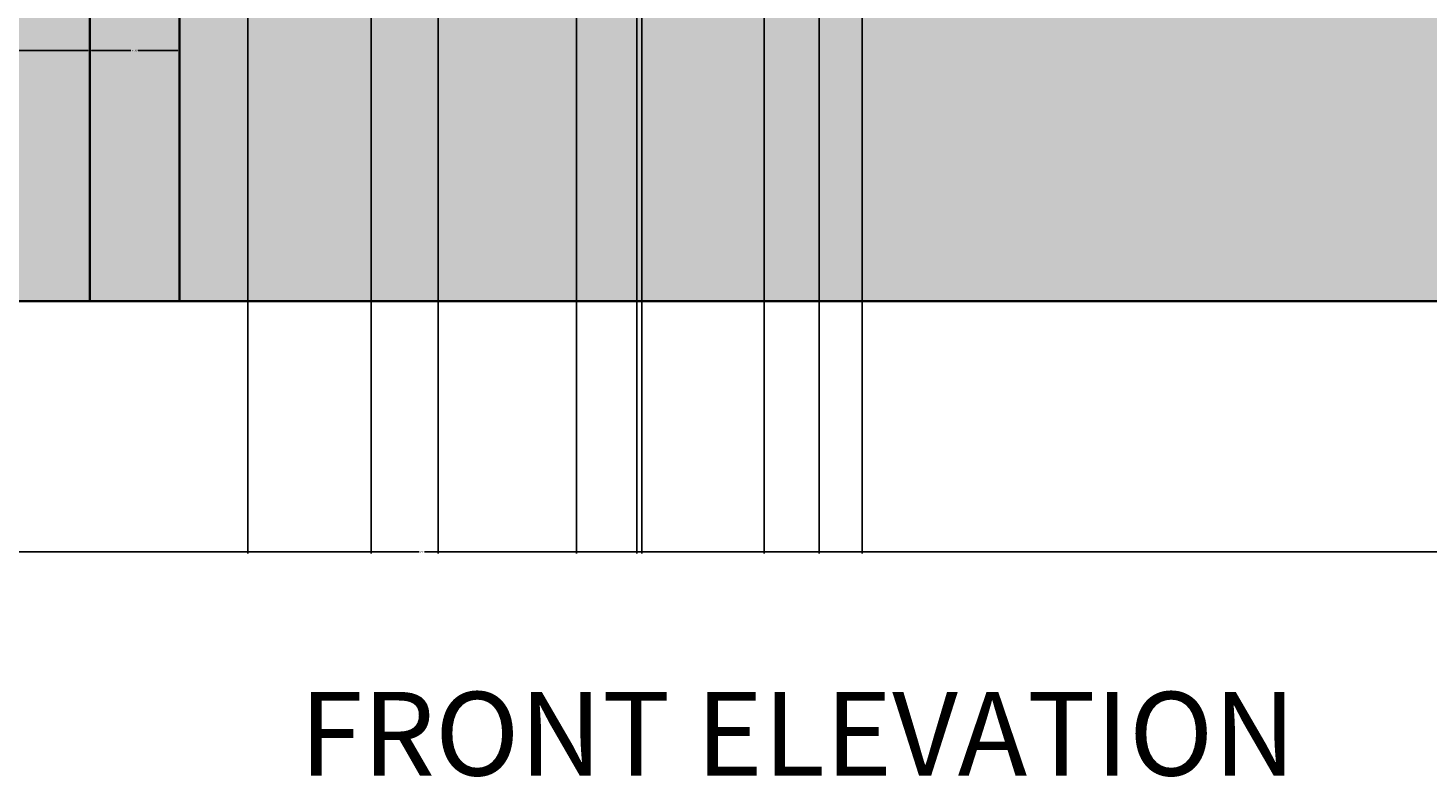
# Model space of a CAD drawing. Units: inches. Extents: x 73 to 607, y 92 to 651.
# Tile 2 of 18: x 298 to 448, y 92 to 173. Entities that reach past the tile are written whole.
import ezdxf

# ---------------------------------------------------------------- set-up
doc = ezdxf.new("R2010")
doc.units = ezdxf.units.IN
doc.header["$MEASUREMENT"] = 0
for name, color, linetype, lineweight in [('A-ANNO-DIMS', 2, 'Continuous', 18), ('A-ANNO-TEXT', 7, 'Continuous', 25), ('A-ELEV', 7, 'Continuous', 35), ('A-ELEV-PATT-WALL', 254, 'Continuous', 13), ('A-ELEV-PATT-WOOD', 32, 'Continuous', 13)]:
    doc.layers.add(name, color=color, linetype=linetype, lineweight=lineweight)
doc.styles.get("Standard").update_dxf_attribs({"font": 'arial.ttf'})
doc.dimstyles.get("Standard").update_dxf_attribs({"dimtxt": 0.18, "dimasz": 0.18, "dimexe": 0.18, "dimexo": 0.0625, "dimgap": 0.09, "dimtad": 0, "dimtih": 1, "dimtoh": 1, "dimdec": 4, "dimzin": 0, "dimdsep": 46, "dimtxsty": 'Standard', "dimcen": 0.09, "dimadec": 0, "dimazin": 0, "dimtfac": 1, "dimtdec": 4, "dimtofl": 0, "dimtmove": 0, "dimatfit": 3, "dimfxl": 1, "dimtolj": 1, "dimtzin": 0, "dimarcsym": 0})

# ---------------------------------------------------------------- blocks, each defined once
blk = doc.blocks.new('*D4')
at = {"layer": 'A-ANNO-DIMS', "color": 0, "lineweight": -2, "transparency": 16777216}
for p, q in [((100.1, 143.14), (100.1, 116.02)), ((580.1, 143.14), (580.1, 116.02)), ((100.28, 116.2), (339.81, 116.2)), ((579.92, 116.2), (340.39, 116.2))]:
    blk.add_line(p, q, dxfattribs=at)
at = {"layer": 'A-ANNO-DIMS', "color": 0, "transparency": 16777216}
for points in [[(100.28, 116.23), (100.28, 116.17), (100.1, 116.2)], [(579.92, 116.23), (579.92, 116.17), (580.1, 116.2)]]:
    blk.add_solid(points, dxfattribs=at)
at = {"layer": 'Defpoints', "color": 0, "transparency": 16777216}
for p in [(100.1, 143.2), (580.1, 143.2), (580.1, 116.2)]:
    blk.add_point(p, dxfattribs=at)
at = {"layer": 'A-ANNO-DIMS', "color": 0, "transparency": 16777216, "insert": (340.1, 116.2), "char_height": 0.18, "attachment_point": 5}
blk.add_mtext('\\A1;480', dxfattribs=at)
blk = doc.blocks.new('*D31')
at = {"layer": 'A-ANNO-DIMS', "color": 0, "lineweight": -2, "transparency": 16777216}
for p, q in [((256.47, 143.27), (256.47, 170.38)), ((304.36, 143.27), (304.36, 170.38)), ((256.65, 170.2), (280.02, 170.2)), ((304.18, 170.2), (280.81, 170.2))]:
    blk.add_line(p, q, dxfattribs=at)
at = {"layer": 'A-ANNO-DIMS', "color": 0, "transparency": 16777216}
for points in [[(256.65, 170.23), (256.65, 170.17), (256.47, 170.2)], [(304.18, 170.23), (304.18, 170.17), (304.36, 170.2)]]:
    blk.add_solid(points, dxfattribs=at)
at = {"layer": 'Defpoints', "color": 0, "transparency": 16777216}
for p in [(304.36, 170.2), (256.47, 143.2), (304.36, 143.2)]:
    blk.add_point(p, dxfattribs=at)
at = {"layer": 'A-ANNO-DIMS', "color": 0, "transparency": 16777216, "insert": (280.41, 170.2), "char_height": 0.18, "attachment_point": 5}
blk.add_mtext('\\A1;47.88', dxfattribs=at)
blk = doc.blocks.new('*D32')
at = {"layer": 'A-ANNO-DIMS', "color": 0, "lineweight": -2, "transparency": 16777216}
for p, q in [((304.36, 143.27), (304.36, 170.38)), ((314.01, 143.27), (314.01, 170.38)), ((304.54, 170.2), (308.79, 170.2)), ((313.83, 170.2), (309.58, 170.2))]:
    blk.add_line(p, q, dxfattribs=at)
at = {"layer": 'A-ANNO-DIMS', "color": 0, "transparency": 16777216}
for points in [[(304.54, 170.23), (304.54, 170.17), (304.36, 170.2)], [(313.83, 170.23), (313.83, 170.17), (314.01, 170.2)]]:
    blk.add_solid(points, dxfattribs=at)
at = {"layer": 'Defpoints', "color": 0, "transparency": 16777216}
for p in [(314.01, 170.2), (304.36, 143.2), (314.01, 143.2)]:
    blk.add_point(p, dxfattribs=at)
at = {"layer": 'A-ANNO-DIMS', "color": 0, "transparency": 16777216, "insert": (309.19, 170.2), "char_height": 0.18, "attachment_point": 5}
blk.add_mtext('\\A1;9.659', dxfattribs=at)
blk = doc.blocks.new('*D77')
at = {"layer": 'A-ANNO-DIMS', "color": 0, "lineweight": -2, "transparency": 16777216}
for p, q in [((321.37, 356.99), (321.37, 116.02)), ((334.67, 320.14), (334.67, 116.02)), ((321.55, 116.2), (327.63, 116.2)), ((334.49, 116.2), (328.4, 116.2))]:
    blk.add_line(p, q, dxfattribs=at)
at = {"layer": 'A-ANNO-DIMS', "color": 0, "transparency": 16777216}
for points in [[(321.55, 116.23), (321.55, 116.17), (321.37, 116.2)], [(334.49, 116.23), (334.49, 116.17), (334.67, 116.2)]]:
    blk.add_solid(points, dxfattribs=at)
at = {"layer": 'Defpoints', "color": 0, "transparency": 16777216}
for p in [(321.37, 357.06), (334.67, 320.2), (321.37, 116.2)]:
    blk.add_point(p, dxfattribs=at)
at = {"layer": 'A-ANNO-DIMS', "color": 0, "transparency": 16777216, "insert": (328.02, 116.2), "char_height": 0.18, "attachment_point": 5}
blk.add_mtext('\\A1;13.30', dxfattribs=at)
blk = doc.blocks.new('*D86')
at = {"layer": 'A-ANNO-DIMS', "color": 0, "lineweight": -2, "transparency": 16777216}
for p, q in [((356.77, 212.97), (356.77, 116.02)), ((341.87, 194.47), (341.87, 116.02)), ((342.05, 116.2), (348.87, 116.2)), ((356.59, 116.2), (349.78, 116.2))]:
    blk.add_line(p, q, dxfattribs=at)
at = {"layer": 'A-ANNO-DIMS', "color": 0, "transparency": 16777216}
for points in [[(342.05, 116.23), (342.05, 116.17), (341.87, 116.2)], [(356.59, 116.23), (356.59, 116.17), (356.77, 116.2)]]:
    blk.add_solid(points, dxfattribs=at)
at = {"layer": 'Defpoints', "color": 0, "transparency": 16777216}
for p in [(356.77, 213.03), (341.87, 194.54), (356.77, 116.2)]:
    blk.add_point(p, dxfattribs=at)
at = {"layer": 'A-ANNO-DIMS', "color": 0, "transparency": 16777216, "insert": (349.32, 116.2), "char_height": 0.18, "attachment_point": 5}
blk.add_mtext('\\A1;14.906', dxfattribs=at)
blk = doc.blocks.new('*D87')
at = {"layer": 'A-ANNO-DIMS', "color": 0, "lineweight": -2, "transparency": 16777216}
for p, q in [((356.77, 212.97), (356.77, 116.02)), ((363.26, 199.09), (363.26, 116.02)), ((356.95, 116.2), (359.62, 116.2)), ((363.08, 116.2), (360.41, 116.2))]:
    blk.add_line(p, q, dxfattribs=at)
at = {"layer": 'A-ANNO-DIMS', "color": 0, "transparency": 16777216}
for points in [[(356.95, 116.23), (356.95, 116.17), (356.77, 116.2)], [(363.08, 116.23), (363.08, 116.17), (363.26, 116.2)]]:
    blk.add_solid(points, dxfattribs=at)
at = {"layer": 'Defpoints', "color": 0, "transparency": 16777216}
for p in [(356.77, 213.03), (363.26, 199.15), (363.26, 116.2)]:
    blk.add_point(p, dxfattribs=at)
at = {"layer": 'A-ANNO-DIMS', "color": 0, "transparency": 16777216, "insert": (360.02, 116.2), "char_height": 0.18, "attachment_point": 5}
blk.add_mtext('\\A1;6.482', dxfattribs=at)
blk = doc.blocks.new('*D88')
at = {"layer": 'A-ANNO-DIMS', "color": 0, "lineweight": -2, "transparency": 16777216}
for p, q in [((376.96, 209.08), (376.96, 116.02)), ((363.26, 199.09), (363.26, 116.02)), ((363.44, 116.2), (369.65, 116.2)), ((376.78, 116.2), (370.56, 116.2))]:
    blk.add_line(p, q, dxfattribs=at)
at = {"layer": 'A-ANNO-DIMS', "color": 0, "transparency": 16777216}
for points in [[(363.44, 116.23), (363.44, 116.17), (363.26, 116.2)], [(376.78, 116.23), (376.78, 116.17), (376.96, 116.2)]]:
    blk.add_solid(points, dxfattribs=at)
at = {"layer": 'Defpoints', "color": 0, "transparency": 16777216}
for p in [(376.96, 209.14), (363.26, 199.15), (376.96, 116.2)]:
    blk.add_point(p, dxfattribs=at)
at = {"layer": 'A-ANNO-DIMS', "color": 0, "transparency": 16777216, "insert": (370.11, 116.2), "char_height": 0.18, "attachment_point": 5}
blk.add_mtext('\\A1;13.704', dxfattribs=at)
blk = doc.blocks.new('*D89')
at = {"layer": 'A-ANNO-DIMS', "color": 0, "lineweight": -2, "transparency": 16777216}
for p, q in [((382.89, 222.03), (382.89, 116.02)), ((376.96, 209.08), (376.96, 116.02)), ((377.14, 116.2), (379.53, 116.2)), ((382.71, 116.2), (380.32, 116.2))]:
    blk.add_line(p, q, dxfattribs=at)
at = {"layer": 'A-ANNO-DIMS', "color": 0, "transparency": 16777216}
for points in [[(377.14, 116.23), (377.14, 116.17), (376.96, 116.2)], [(382.71, 116.23), (382.71, 116.17), (382.89, 116.2)]]:
    blk.add_solid(points, dxfattribs=at)
at = {"layer": 'Defpoints', "color": 0, "transparency": 16777216}
for p in [(382.89, 222.1), (376.96, 209.14), (382.89, 116.2)]:
    blk.add_point(p, dxfattribs=at)
at = {"layer": 'A-ANNO-DIMS', "color": 0, "transparency": 16777216, "insert": (379.92, 116.2), "char_height": 0.18, "attachment_point": 5}
blk.add_mtext('\\A1;5.926', dxfattribs=at)
blk = doc.blocks.new('*D90')
at = {"layer": 'A-ANNO-DIMS', "color": 0, "lineweight": -2, "transparency": 16777216}
for p, q in [((382.89, 222.03), (382.89, 116.02)), ((387.52, 200.01), (387.52, 116.02)), ((383.07, 116.2), (384.87, 116.2)), ((387.34, 116.2), (385.53, 116.2))]:
    blk.add_line(p, q, dxfattribs=at)
at = {"layer": 'A-ANNO-DIMS', "color": 0, "transparency": 16777216}
for points in [[(383.07, 116.23), (383.07, 116.17), (382.89, 116.2)], [(387.34, 116.23), (387.34, 116.17), (387.52, 116.2)]]:
    blk.add_solid(points, dxfattribs=at)
at = {"layer": 'Defpoints', "color": 0, "transparency": 16777216}
for p in [(382.89, 222.1), (387.52, 200.08), (387.52, 116.2)]:
    blk.add_point(p, dxfattribs=at)
at = {"layer": 'A-ANNO-DIMS', "color": 0, "transparency": 16777216, "insert": (385.2, 116.2), "char_height": 0.18, "attachment_point": 5}
blk.add_mtext('\\A1;4.63', dxfattribs=at)
blk = doc.blocks.new('*D91')
at = {"layer": 'A-ANNO-DIMS', "color": 0, "lineweight": -2, "transparency": 16777216}
for p, q in [((363.81, 225.92), (363.81, 116.02)), ((356.77, 212.97), (356.77, 116.02)), ((356.95, 116.2), (359.9, 116.2)), ((363.63, 116.2), (360.69, 116.2))]:
    blk.add_line(p, q, dxfattribs=at)
at = {"layer": 'A-ANNO-DIMS', "color": 0, "transparency": 16777216}
for points in [[(356.95, 116.23), (356.95, 116.17), (356.77, 116.2)], [(363.63, 116.23), (363.63, 116.17), (363.81, 116.2)]]:
    blk.add_solid(points, dxfattribs=at)
at = {"layer": 'Defpoints', "color": 0, "transparency": 16777216}
for p in [(363.81, 225.98), (356.77, 213.03), (363.81, 116.2)]:
    blk.add_point(p, dxfattribs=at)
at = {"layer": 'A-ANNO-DIMS', "color": 0, "transparency": 16777216, "insert": (360.29, 116.2), "char_height": 0.18, "attachment_point": 5}
blk.add_mtext('\\A1;7.037', dxfattribs=at)

msp = doc.modelspace()

# ---------------------------------------------------------------- hatches: boundary and pattern name
at = {"layer": 'A-ELEV-PATT-WALL'}
h = msp.add_hatch(color=256, dxfattribs=at)
h.dxf.hatch_style = 1
h.paths.add_polyline_path([(509.9692, 483.857), (450.6603, 483.857), (450.6603, 465.0632), (446.1603, 465.0632), (446.1603, 484.2142), (374.4727, 484.2142), (374.4727, 465.0632), (369.9727, 465.0632), (369.9727, 484.2142), (321.3008, 484.2142), (321.3008, 412.636), (451.5214, 412.636), (451.5214, 311.2042), (314.0144, 311.2042), (314.0144, 253.4054), (347.8686, 253.4054), (347.8686, 247.4054), (369.5339, 247.4054), (369.5339, 258.6914), (431.07, 258.6914), (431.07, 185.6619), (369.5339, 185.6619), (369.5339, 194.5366), (347.8686, 194.5366), (347.8686, 188.5452), (314.0144, 188.5452), (314.0144, 143.2042), (451.5214, 143.2042), (451.5214, 262.3024), (580.0983, 262.3024), (580.0983, 311.2042), (509.9692, 311.2042)])
h.paths.add_polyline_path([(304.3559, 311.2042), (256.4726, 311.2042), (256.4726, 167.2042), (256.4726, 143.2042), (304.3559, 143.2042), (304.3559, 188.5452), (298.3559, 188.5452), (298.3559, 253.4054), (304.3559, 253.4054)])
at = {"layer": 'A-ELEV-PATT-WOOD'}
h = msp.add_hatch(color=256, dxfattribs=at)
h.dxf.hatch_style = 1
h.paths.add_polyline_path([(314.0144, 311.2042), (304.3559, 311.2042), (304.3559, 143.2042), (314.0144, 143.2042)])

# ---------------------------------------------------------------- linework, layer by layer
at = {"layer": 'A-ELEV'}
msp.add_line((100.0983, 143.2042), (580.0983, 143.2042), dxfattribs=at)
msp.add_lwpolyline([(304.3559, 143.2042), (314.0144, 143.2042), (314.0144, 311.2042), (304.3559, 311.2042)], close=True, dxfattribs=at)

# ---------------------------------------------------------------- texts
at = {"layer": 'A-ANNO-TEXT', "insert": (326.9467, 101.1273), "char_height": 9, "attachment_point": 1}
msp.add_mtext_dynamic_manual_height_columns('FRONT ELEVATION', width=214.95561, gutter_width=1, heights=[0], dxfattribs=at)

# ---------------------------------------------------------------- dimensions: what is measured, and where the dimension line sits
at = {"layer": 'A-ANNO-DIMS'}
for base, p1, p2, override, picture, middle in [((321.3681, 116.2042), (334.6695, 320.2042), (321.3681, 357.0571), {"dimdec": 2, "dimlfac": 1, "dimrnd": 0, "dimzin": 0, "dimdsep": 46, "dimlunit": 2}, '*D77', (328.0188, 116.2042)), ((363.8119, 116.2042), (356.7748, 213.0292), (363.8119, 225.982), {"dimdec": 3, "dimlfac": 1, "dimrnd": 0, "dimzin": 0, "dimdsep": 46, "dimlunit": 2}, '*D91', (360.2933, 116.2042)), ((382.8864, 116.2042), (376.9603, 209.1433), (382.8864, 222.0962), {"dimdec": 3, "dimlfac": 1, "dimrnd": 0, "dimzin": 0, "dimdsep": 46, "dimlunit": 2}, '*D89', (379.9234, 116.2042)), ((387.5161, 116.2042), (382.8864, 222.0962), (387.5161, 200.0764), {"dimdec": 2, "dimlfac": 1, "dimrnd": 0, "dimzin": 0, "dimdsep": 46, "dimlunit": 2}, '*D90', (385.2013, 116.2042)), ((356.7748, 116.2042), (341.8686, 194.5366), (356.7748, 213.0292), {"dimdec": 3, "dimlfac": 1, "dimrnd": 0, "dimzin": 0, "dimdsep": 46, "dimlunit": 2}, '*D86', (349.3217, 116.2042)), ((363.2564, 116.2042), (356.7748, 213.0292), (363.2564, 199.1512), {"dimdec": 3, "dimlfac": 1, "dimrnd": 0, "dimzin": 0, "dimdsep": 46, "dimlunit": 2}, '*D87', (360.0156, 116.2042)), ((376.9603, 116.2042), (363.2564, 199.1512), (376.9603, 209.1433), {"dimdec": 3, "dimlfac": 1, "dimrnd": 0, "dimzin": 0, "dimdsep": 46, "dimlunit": 2}, '*D88', (370.1084, 116.2042)), ((304.3559, 170.2042), (256.4726, 143.2042), (304.3559, 143.2042), {"dimdec": 2, "dimlfac": 1, "dimrnd": 0, "dimzin": 0, "dimdsep": 46, "dimlunit": 2}, '*D31', (280.4142, 170.2042)), ((314.01441, 170.2042), (304.35586, 143.2042), (314.01441, 143.2042), {"dimdec": 3, "dimlfac": 1, "dimrnd": 0, "dimzin": 0, "dimdsep": 46, "dimlunit": 2}, '*D32', (309.18514, 170.2042)), ((580.0983, 116.2042), (100.0983, 143.2042), (580.0983, 143.2042), {"dimdec": 0, "dimlfac": 1, "dimrnd": 0, "dimzin": 0, "dimdsep": 46, "dimlunit": 2}, '*D4', (340.0983, 116.2042))]:
    dim = msp.add_linear_dim(base=base, p1=p1, p2=p2, dimstyle='Standard', override=override, dxfattribs=at)
    dim.commit()
    dim.dimension.update_dxf_attribs({"geometry": picture, "text_midpoint": middle})

doc.saveas('drawing.dxf')
